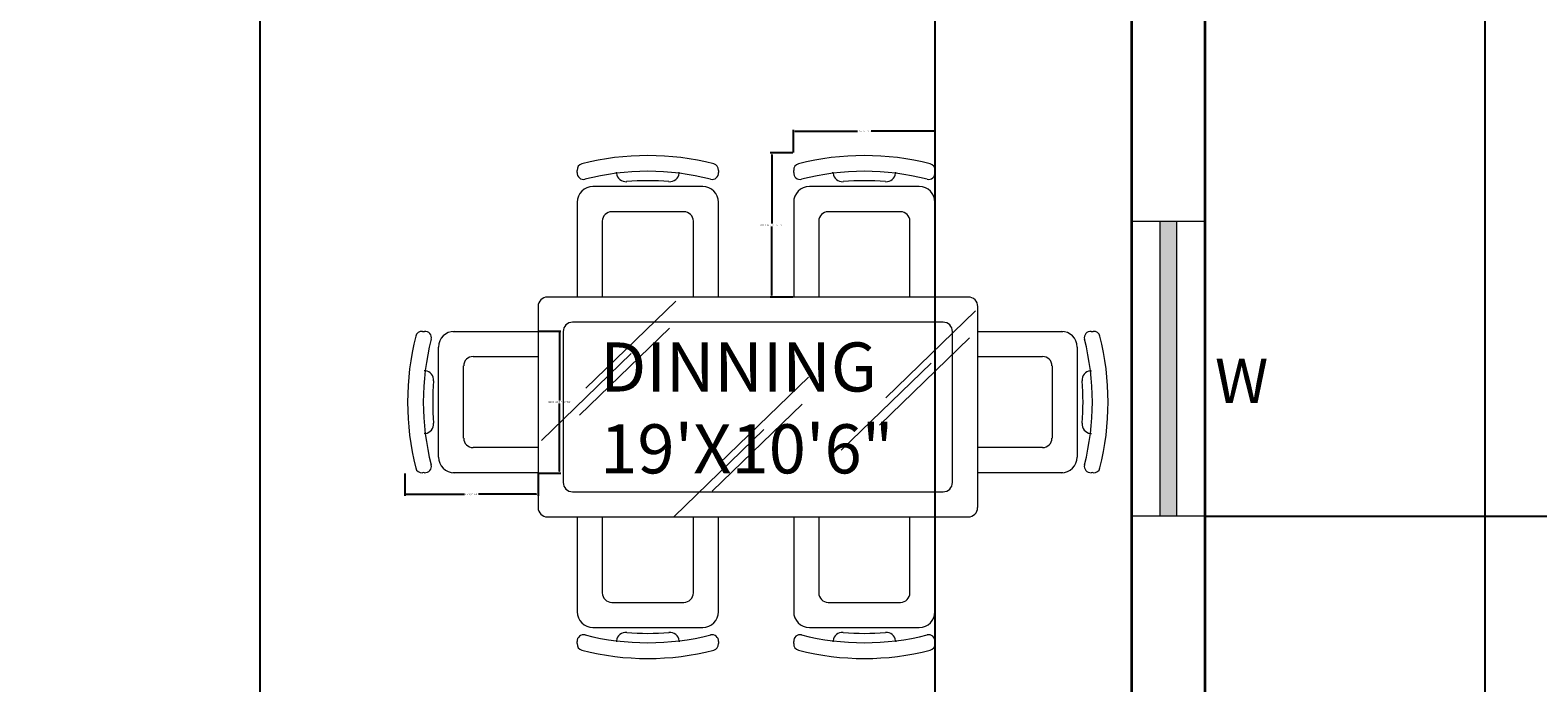
# Model space of a CAD drawing. Units: inches. Extents: x 502 to 1235, y -850 to 110.
# Tile 4 of 9: x 867 to 1051, y -415 to -335. Entities that reach past the tile are written whole.
import ezdxf

# ---------------------------------------------------------------- set-up
doc = ezdxf.new("R2010")
doc.units = ezdxf.units.IN
doc.header["$MEASUREMENT"] = 0
for name, color, linetype, lineweight in [('A-ANNO-DIMS', 2, 'Continuous', 18), ('A-ANNO-TEXT', 7, 'Continuous', 18), ('A-AREA-IDEN', 8, 'Continuous', 18), ('A-GLAZ-PATT', 5, 'Continuous', 13), ('WALL', 1, 'Continuous', 35), ('WIN', 5, 'Continuous', 18)]:
    doc.layers.add(name, color=color, linetype=linetype, lineweight=lineweight)
doc.layers.add('furniture', color=50, linetype='Continuous', lineweight=13, transparency=0.8)
doc.styles.get("Standard").update_dxf_attribs({"font": 'arial.ttf'})
doc.dimstyles.get("Standard").update_dxf_attribs({"dimtxt": 0.18, "dimasz": 0.18, "dimexe": 0.18, "dimexo": 0.0625, "dimgap": 0.09, "dimtad": 0, "dimtih": 1, "dimtoh": 1, "dimdec": 1, "dimzin": 0, "dimdsep": 46, "dimlunit": 4, "dimtxsty": 'Standard', "dimcen": 0.09, "dimadec": 0, "dimazin": 0, "dimtfac": 1, "dimtdec": 1, "dimtofl": 0, "dimtmove": 0, "dimatfit": 3, "dimfxl": 1, "dimtolj": 1, "dimtzin": 0, "dimarcsym": 0})

# ---------------------------------------------------------------- blocks, each defined once
blk = doc.blocks.new('_ArchTick')
at = {"color": 0, "linetype": 'ByBlock', "const_width": 0.15}
blk.add_lwpolyline([(-0.5, -0.5), (0.5, 0.5)], dxfattribs=at)
blk = doc.blocks.new('*D7')
at = {"layer": 'A-ANNO-DIMS', "color": 0, "lineweight": -2, "transparency": 16777216}
for p, q in [((1043.54, -60.85), (1044.72, -60.85)), ((1044.54, -60.85), (1044.54, -551.48)), ((1043.54, -551.48), (1044.72, -551.48))]:
    blk.add_line(p, q, dxfattribs=at)
at = {"layer": 'Defpoints', "color": 0, "transparency": 16777216}
for p in [(1010.39, -60.85), (1010.39, -551.48), (1044.54, -551.48)]:
    blk.add_point(p, dxfattribs=at)
at = {"layer": 'A-ANNO-DIMS', "color": 0, "lineweight": -2, "transparency": 16777216, "xscale": 5, "yscale": 5, "zscale": 5}
for p, rotation in [((1044.54, -60.85), 90), ((1044.54, -551.48), 270)]:
    blk.add_blockref('_ArchTick', p, dxfattribs=dict(at, rotation=rotation))
at = {"layer": 'A-ANNO-DIMS', "color": 0, "transparency": 16777216, "insert": (1036.52, -306.16), "char_height": 8, "attachment_point": 5, "rotation": 90}
blk.add_mtext("\\A1;42'", dxfattribs=at)
blk = doc.blocks.new('WIN-36IN')
for p, q in [((0, 0), (0, 9)), ((36, 0), (36, 9)), ((0, 5.5), (36, 5.5)), ((0, 3.5), (36, 3.5))]:
    blk.add_line(p, q)
blk = doc.blocks.new('CHAIR-DINING-SIDE')
for p, q in [((4.8, 15.13), (4.8, 15.25)), ((12.47, 15.13), (12.47, 15.25)), ((15.35, 13.5), (1.92, 13.5)), ((0, 11.76), (0, 11.36)), ((0, 11.58), (0, 0)), ((17.27, 11.36), (17.27, 11.76)), ((17.27, 0), (17.27, 11.58)), ((3.07, 9.28), (3.07, 0)), ((13.05, 10.43), (4.22, 10.43)), ((14.2, 0), (14.2, 9.28))]:
    blk.add_line(p, q)
for centre, radius, start, end in [((8.63, -15.67), 32.96, 75.853, 104.147), ((0.77, 15.54), 0.768, 104.147, 185.9216), ((-1.14, 15.34), 1.15, 354.0784, 5.9216), ((0.77, 15.15), 0.768, 174.0784, 284.3214), ((8.63, -15.67), 31.04, 75.6786, 104.3214), ((5.95, 15.25), 1.15, 186.0281, 274.9654), ((11.32, 15.25), 1.15, 265.0346, 353.9719), ((16.5, 15.15), 0.768, 255.6786, 5.9216), ((16.5, 15.54), 0.768, 354.0784, 75.853), ((18.41, 15.34), 1.15, 174.0784, 185.9216), ((1.92, 11.58), 1.92, 90, 180), ((8.63, -15.67), 29.89, 85.0346, 94.9654), ((15.35, 11.58), 1.92, 0, 90), ((4.22, 9.28), 1.15, 90, 180), ((13.05, 9.28), 1.15, 0, 90)]:
    blk.add_arc(centre, radius, start, end)
blk = doc.blocks.new('CHAIR-DINING-END')
for p, q in [((5.53, 17.27), (5.92, 17.27)), ((5.7, 17.27), (15.95, 17.27)), ((3.78, 1.92), (3.78, 15.35)), ((6.85, 4.22), (6.85, 13.05)), ((8.01, 14.2), (15.95, 14.2)), ((2.16, 12.47), (2.04, 12.47)), ((2.16, 4.8), (2.04, 4.8)), ((15.95, 3.07), (8.01, 3.07)), ((5.92, 0), (5.53, 0)), ((15.95, 0), (5.7, 0))]:
    blk.add_line(p, q)
for centre, radius, start, end in [((32.96, 8.63), 32.96, 165.853, 194.147), ((1.74, 16.5), 0.768, 84.0784, 165.853), ((1.94, 18.41), 1.15, 264.0784, 275.9216), ((2.14, 16.5), 0.768, 345.6786, 95.9216), ((5.7, 15.35), 1.92, 90, 180), ((32.96, 8.63), 31.04, 165.6786, 194.3214), ((8.01, 13.05), 1.15, 90, 180), ((2.04, 11.32), 1.15, 355.0346, 83.9719), ((32.96, 8.63), 29.89, 175.0346, 184.9654), ((2.04, 5.95), 1.15, 276.0281, 4.9654), ((8.01, 4.22), 1.15, 180, 270), ((5.7, 1.92), 1.92, 180, 270), ((1.74, 0.77), 0.768, 194.147, 275.9216), ((1.94, -1.14), 1.15, 84.0784, 95.9216), ((2.14, 0.77), 0.768, 264.0784, 14.3214)]:
    blk.add_arc(centre, radius, start, end)
blk = doc.blocks.new('*D18')
at = {"layer": 'A-ANNO-DIMS', "color": 0, "lineweight": -2, "transparency": 16777216}
for p, q in [((959.98, -350.46), (957.22, -350.46)), ((957.4, -350.64), (957.4, -359.09)), ((957.4, -367.9), (957.4, -359.46)), ((959.98, -368.08), (957.22, -368.08))]:
    blk.add_line(p, q, dxfattribs=at)
at = {"layer": 'A-ANNO-DIMS', "color": 0, "transparency": 16777216}
for points in [[(957.37, -350.64), (957.43, -350.64), (957.4, -350.46)], [(957.37, -367.9), (957.43, -367.9), (957.4, -368.08)]]:
    blk.add_solid(points, dxfattribs=at)
at = {"layer": 'Defpoints', "color": 0, "transparency": 16777216}
for p in [(957.4, -350.46), (960.04, -350.46), (960.04, -368.08)]:
    blk.add_point(p, dxfattribs=at)
at = {"layer": 'A-ANNO-DIMS', "color": 0, "transparency": 16777216, "insert": (957.4, -359.27), "char_height": 0.18, "attachment_point": 5}
blk.add_mtext('\\A1;SIDE CHAIR 1\'-5 1/2" TYP.', dxfattribs=at)
blk = doc.blocks.new('*D19')
at = {"layer": 'A-ANNO-DIMS', "color": 0, "lineweight": -2, "transparency": 16777216}
for p, q in [((960.04, -350.4), (960.04, -347.64)), ((960.22, -347.82), (967.87, -347.82)), ((977.2, -347.82), (969.55, -347.82)), ((977.38, -350.4), (977.38, -347.64))]:
    blk.add_line(p, q, dxfattribs=at)
at = {"layer": 'A-ANNO-DIMS', "color": 0, "transparency": 16777216}
for points in [[(960.22, -347.79), (960.22, -347.85), (960.04, -347.82)], [(977.2, -347.79), (977.2, -347.85), (977.38, -347.82)]]:
    blk.add_solid(points, dxfattribs=at)
at = {"layer": 'Defpoints', "color": 0, "transparency": 16777216}
for p in [(977.38, -347.82), (960.04, -350.46), (977.38, -350.46)]:
    blk.add_point(p, dxfattribs=at)
at = {"layer": 'A-ANNO-DIMS', "color": 0, "transparency": 16777216, "insert": (968.71, -347.82), "char_height": 0.18, "attachment_point": 5}
blk.add_mtext('\\A1;1\'-5 1/2" TYP.', dxfattribs=at)
blk = doc.blocks.new('*D20')
at = {"layer": 'A-ANNO-DIMS', "color": 0, "lineweight": -2, "transparency": 16777216}
for p, q in [((928.9, -372.24), (931.62, -372.24)), ((931.44, -372.42), (931.44, -380.73)), ((931.44, -389.4), (931.44, -381.09)), ((928.9, -389.58), (931.62, -389.58))]:
    blk.add_line(p, q, dxfattribs=at)
at = {"layer": 'A-ANNO-DIMS', "color": 0, "transparency": 16777216}
for points in [[(931.41, -372.42), (931.47, -372.42), (931.44, -372.24)], [(931.41, -389.4), (931.47, -389.4), (931.44, -389.58)]]:
    blk.add_solid(points, dxfattribs=at)
at = {"layer": 'Defpoints', "color": 0, "transparency": 16777216}
for p in [(928.84, -372.24), (931.44, -372.24), (928.84, -389.58)]:
    blk.add_point(p, dxfattribs=at)
at = {"layer": 'A-ANNO-DIMS', "color": 0, "transparency": 16777216, "insert": (931.44, -380.91), "char_height": 0.18, "attachment_point": 5}
blk.add_mtext('\\A1;END CHAIR 1\'-5 1/2" TYP.', dxfattribs=at)
blk = doc.blocks.new('*D21')
at = {"layer": 'A-ANNO-DIMS', "color": 0, "lineweight": -2, "transparency": 16777216}
for p, q in [((912.56, -389.64), (912.56, -392.36)), ((928.84, -389.64), (928.84, -392.36)), ((912.74, -392.18), (919.86, -392.18)), ((928.66, -392.18), (921.54, -392.18))]:
    blk.add_line(p, q, dxfattribs=at)
at = {"layer": 'A-ANNO-DIMS', "color": 0, "transparency": 16777216}
for points in [[(912.74, -392.15), (912.74, -392.21), (912.56, -392.18)], [(928.66, -392.15), (928.66, -392.21), (928.84, -392.18)]]:
    blk.add_solid(points, dxfattribs=at)
at = {"layer": 'Defpoints', "color": 0, "transparency": 16777216}
for p in [(912.56, -389.58), (928.84, -389.58), (928.84, -392.18)]:
    blk.add_point(p, dxfattribs=at)
at = {"layer": 'A-ANNO-DIMS', "color": 0, "transparency": 16777216, "insert": (920.7, -392.18), "char_height": 0.18, "attachment_point": 5}
blk.add_mtext('\\A1;1\'-4 1/2" TYP.', dxfattribs=at)
blk = doc.blocks.new('*D25')
at = {"layer": 'A-ANNO-DIMS', "color": 0, "lineweight": -2, "transparency": 16777216}
for p, q in [((798.89, -699.78), (798.89, 63.98)), ((799.07, 63.8), (846.56, 63.8)), ((894.71, 63.8), (847.22, 63.8)), ((894.89, -699.78), (894.89, 63.98))]:
    blk.add_line(p, q, dxfattribs=at)
at = {"layer": 'A-ANNO-DIMS', "color": 0, "transparency": 16777216}
for points in [[(799.07, 63.83), (799.07, 63.77), (798.89, 63.8)], [(894.71, 63.83), (894.71, 63.77), (894.89, 63.8)]]:
    blk.add_solid(points, dxfattribs=at)
at = {"layer": 'Defpoints', "color": 0, "transparency": 16777216}
for p in [(894.89, 63.8), (798.89, -699.85), (894.89, -699.85)]:
    blk.add_point(p, dxfattribs=at)
at = {"layer": 'A-ANNO-DIMS', "color": 0, "transparency": 16777216, "insert": (846.89, 63.8), "char_height": 0.18, "attachment_point": 5}
blk.add_mtext('\\A1;8\'-0"', dxfattribs=at)
blk = doc.blocks.new('*D43')
at = {"layer": 'A-ANNO-DIMS', "color": 0, "lineweight": -2, "transparency": 16777216}
for p, q in [((977.39, -422.28), (977.39, 63.98)), ((977.57, 63.8), (989.06, 63.8)), ((1001.21, 63.8), (989.72, 63.8)), ((1001.39, -422.28), (1001.39, 63.98))]:
    blk.add_line(p, q, dxfattribs=at)
at = {"layer": 'A-ANNO-DIMS', "color": 0, "transparency": 16777216}
for points in [[(977.57, 63.83), (977.57, 63.77), (977.39, 63.8)], [(1001.21, 63.83), (1001.21, 63.77), (1001.39, 63.8)]]:
    blk.add_solid(points, dxfattribs=at)
at = {"layer": 'Defpoints', "color": 0, "transparency": 16777216}
for p in [(1001.39, 63.8), (977.39, -422.35), (1001.39, -422.35)]:
    blk.add_point(p, dxfattribs=at)
at = {"layer": 'A-ANNO-DIMS', "color": 0, "transparency": 16777216, "insert": (989.39, 63.8), "char_height": 0.18, "attachment_point": 5}
blk.add_mtext('\\A1;2\'-0"', dxfattribs=at)
blk = doc.blocks.new('*D55')
at = {"layer": 'A-ANNO-DIMS', "color": 0, "lineweight": -2, "transparency": 16777216}
for p, q in [((1010.45, -394.85), (1235.01, -394.85)), ((1234.83, -395.03), (1234.83, -415.12)), ((1234.83, -435.56), (1234.83, -415.48)), ((1010.45, -435.74), (1235.01, -435.74))]:
    blk.add_line(p, q, dxfattribs=at)
at = {"layer": 'A-ANNO-DIMS', "color": 0, "transparency": 16777216}
for points in [[(1234.8, -395.03), (1234.86, -395.03), (1234.83, -394.85)], [(1234.8, -435.56), (1234.86, -435.56), (1234.83, -435.74)]]:
    blk.add_solid(points, dxfattribs=at)
at = {"layer": 'Defpoints', "color": 0, "transparency": 16777216}
for p in [(1010.39, -394.85), (1234.83, -394.85), (1010.39, -435.74)]:
    blk.add_point(p, dxfattribs=at)
at = {"layer": 'A-ANNO-DIMS', "color": 0, "transparency": 16777216, "insert": (1234.83, -415.3), "char_height": 0.18, "attachment_point": 5}
blk.add_mtext('\\A1;3\'-5"', dxfattribs=at)

msp = doc.modelspace()

# ---------------------------------------------------------------- hatches: boundary and pattern name
at = {"layer": 'A-GLAZ-PATT'}
h = msp.add_hatch(color=256, dxfattribs=at)
h.dxf.hatch_style = 1
h.paths.add_polyline_path([(769.5, -64.35), (769.5, -66.35), (805.5, -66.35), (805.5, -64.35)])
h.paths.add_polyline_path([(845.65, -64.35), (821.65, -64.35), (821.65, -66.35), (845.65, -66.35)])
h.paths.add_polyline_path([(995.07, -64.35), (959.07, -64.35), (959.07, -66.35), (995.07, -66.35)])
h.paths.add_polyline_path([(1006.89, -358.85), (1004.89, -358.85), (1004.89, -394.85), (1006.89, -394.85)])
h.paths.add_polyline_path([(1006.89, -435.74), (1004.89, -435.74), (1004.89, -471.74), (1006.89, -471.74)])
h.paths.add_polyline_path([(874.64, -545.85), (874.64, -547.85), (910.64, -547.85), (910.64, -545.85)])
h.paths.add_polyline_path([(640.89, -310.35), (638.89, -310.35), (638.89, -334.35), (640.89, -334.35)])
h.paths.add_polyline_path([(640.89, -358.06), (638.89, -358.06), (638.89, -394.06), (640.89, -394.06)])

# ---------------------------------------------------------------- linework, layer by layer
at = {"layer": 'furniture'}
for p, q in [((981.41, -368.08), (929.99, -368.08)), ((928.84, -369.23), (928.84, -393.79)), ((945.66, -368.58), (934.68, -379.21)), ((982.32, -369.76), (971.34, -380.39)), ((982.57, -393.79), (982.57, -369.23)), ((978.34, -371.15), (933.06, -371.15)), ((944.9, -371.89), (933.92, -382.52)), ((931.91, -372.3), (931.91, -390.72)), ((981.56, -373.07), (970.58, -383.71)), ((979.5, -390.72), (979.5, -372.3)), ((940.23, -374.98), (929.24, -385.61)), ((976.88, -376.16), (965.9, -386.8)), ((961.88, -377.86), (950.9, -388.49)), ((961.12, -381.17), (950.13, -391.81)), ((956.44, -384.26), (945.46, -394.9)), ((933.06, -391.88), (978.34, -391.88)), ((929.99, -394.95), (981.41, -394.95))]:
    msp.add_line(p, q, dxfattribs=at)
for centre, radius, start, end in [((929.99, -369.23), 1.15, 90, 180), ((981.47, -369.18), 1.1, 357.166, 92.834), ((933.06, -372.3), 1.15, 90, 180), ((978.34, -372.3), 1.15, 0, 90), ((933.06, -390.72), 1.15, 180, 270), ((978.34, -390.72), 1.15, 270, 0), ((929.99, -393.79), 1.15, 180, 270), ((981.41, -393.79), 1.15, 270, 0)]:
    msp.add_arc(centre, radius, start, end, dxfattribs=at)
at = {"layer": 'WALL'}
for p, q in [((1010.39, -615.85), (1010.39, -60.85)), ((1001.39, -418.35), (1001.39, -193.85))]:
    msp.add_line(p, q, dxfattribs=at)

# ---------------------------------------------------------------- block references
at = {"layer": 'furniture'}
for name, p in [('CHAIR-DINING-SIDE', (933.62, -368.08)), ('CHAIR-DINING-SIDE', (960.08, -368.08)), ('CHAIR-DINING-END', (912.89, -389.54))]:
    msp.add_blockref(name, p, dxfattribs=at)
at = {"layer": 'furniture', "rotation": 180}
for name, p in [('CHAIR-DINING-END', (998.51, -372.27)), ('CHAIR-DINING-SIDE', (950.89, -394.95)), ('CHAIR-DINING-SIDE', (977.35, -394.95))]:
    msp.add_blockref(name, p, dxfattribs=at)
at = {"layer": 'WIN', "rotation": 90.00000000000038}
msp.add_blockref('WIN-36IN', (1010.39, -394.85), dxfattribs=at)

# ---------------------------------------------------------------- texts
at = {"layer": 'A-ANNO-TEXT'}
msp.add_text('W', height=5.44, dxfattribs=at).set_placement((1011.57, -381.04))
at = {"layer": 'A-AREA-IDEN', "insert": (929.1, -373.62), "char_height": 6, "attachment_point": 1}
msp.add_mtext_dynamic_manual_height_columns('    DINNING\\P    19\'X10\'6"', width=53.3957, gutter_width=1, heights=[0], dxfattribs=at)

# ---------------------------------------------------------------- dimensions: what is measured, and where the dimension line sits
at = {"layer": 'A-ANNO-DIMS'}
for base, p1, p2, picture, middle in [((894.89, 63.8), (798.89, -699.85), (894.89, -699.85), '*D25', (846.89, 63.8)), ((1001.39, 63.8), (977.39, -422.35), (1001.39, -422.35), '*D43', (989.39, 63.8))]:
    dim = msp.add_linear_dim(base=base, p1=p1, p2=p2, dimstyle='Standard', override={"dimdec": 1, "dimlfac": 1, "dimrnd": 0, "dimzin": 1, "dimdsep": 46, "dimlunit": 4, "dimfrac": 2}, dxfattribs=at)
    dim.commit()
    dim.dimension.update_dxf_attribs({"geometry": picture, "text_midpoint": middle})
for base, p1, p2, text, override, picture, middle in [((1044.54, -551.48), (1010.39, -60.85), (1010.39, -551.48), "42'", {"dimtxt": 8, "dimasz": 5, "dimgap": 4, "dimtad": 1, "dimtih": 0, "dimblk1": 'ArchTick', "dimblk2": 'ArchTick', "dimsah": 1, "dimclrd": 0, "dimclre": 0, "dimclrt": 0, "dimfxlon": 1}, '*D7', (1036.52, -306.16)), ((957.4, -350.46), (960.04, -368.08), (960.04, -350.46), 'SIDE CHAIR <> TYP.', {"dimdec": 1, "dimlfac": 1, "dimrnd": 0, "dimzin": 1, "dimdsep": 46, "dimlunit": 4, "dimfrac": 2}, '*D18', (957.4, -359.27)), ((931.44, -372.24), (928.84, -389.58), (928.84, -372.24), 'END CHAIR <> TYP.', {"dimdec": 1, "dimlfac": 1, "dimrnd": 0, "dimzin": 1, "dimdsep": 46, "dimlunit": 4, "dimfrac": 2}, '*D20', (931.44, -380.91))]:
    dim = msp.add_linear_dim(base=base, p1=p1, p2=p2, angle=90, text=text, dimstyle='Standard', override=override, dxfattribs=at)
    dim.commit()
    dim.dimension.update_dxf_attribs({"geometry": picture, "text_midpoint": middle})
for base, p1, p2, picture, middle in [((977.38, -347.82), (960.04, -350.46), (977.38, -350.46), '*D19', (968.71, -347.82)), ((928.84, -392.18), (912.56, -389.58), (928.84, -389.58), '*D21', (920.7, -392.18))]:
    dim = msp.add_linear_dim(base=base, p1=p1, p2=p2, text='<> TYP.', dimstyle='Standard', override={"dimdec": 1, "dimlfac": 1, "dimrnd": 0, "dimzin": 1, "dimdsep": 46, "dimlunit": 4, "dimfrac": 2}, dxfattribs=at)
    dim.commit()
    dim.dimension.update_dxf_attribs({"geometry": picture, "text_midpoint": middle})
dim = msp.add_linear_dim(base=(1234.83, -394.85), p1=(1010.39, -435.74), p2=(1010.39, -394.85), angle=90, dimstyle='Standard', override={"dimdec": 1, "dimlfac": 1, "dimrnd": 0, "dimzin": 1, "dimdsep": 46, "dimlunit": 4, "dimfrac": 2}, dxfattribs=at)
dim.commit()
dim.dimension.update_dxf_attribs({"geometry": '*D55', "text_midpoint": (1234.83, -415.3)})

doc.saveas('drawing.dxf')
